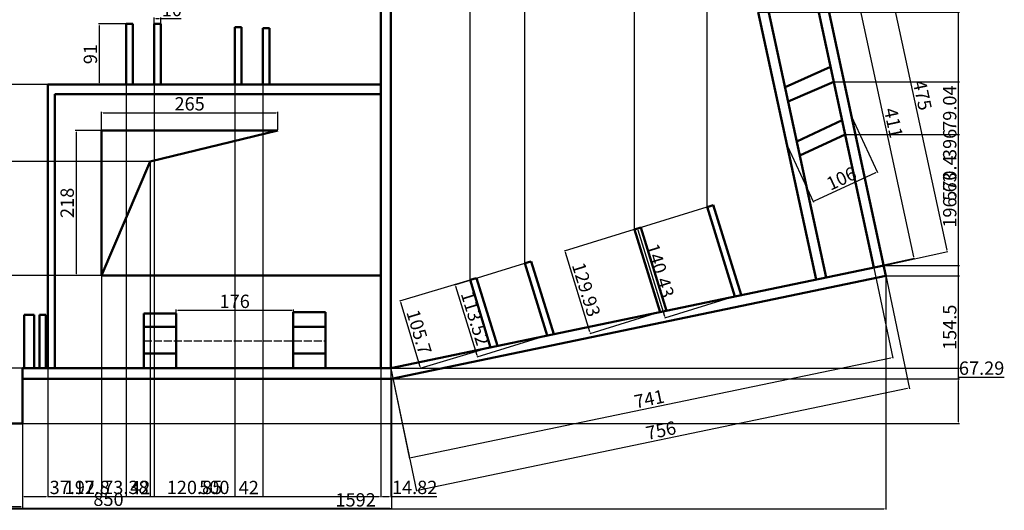
# Model space of a CAD drawing. Units: millimetres. Extents: x 1408 to 3734, y 1022 to 2569.
# Tile 2 of 3: x 2256 to 3734, y 1022 to 1758. Entities that reach past the tile are written whole.
import ezdxf

# ---------------------------------------------------------------- set-up
doc = ezdxf.new("R2010")
doc.units = ezdxf.units.MM
doc.linetypes.add('ACAD_ISO02W100', pattern=[15, 12, -3])
for name, color, linetype, lineweight in [('M-DIMS', 2, 'Continuous', 25), ('M-HIDN', 4, 'ACAD_ISO02W100', 25), ('M-OUTL', 7, 'Continuous', 50)]:
    doc.layers.add(name, color=color, linetype=linetype, lineweight=lineweight)
doc.styles.get("Standard").update_dxf_attribs({"font": 'arial.ttf'})
doc.dimstyles.new('ISO-25', dxfattribs={"dimtxt": 20, "dimasz": 2.5, "dimexe": 1.25, "dimexo": 0.625, "dimtad": 1, "dimtoh": 1, "dimdec": 0, "dimtxsty": 'Standard', "dimcen": 2.5, "dimadec": 0, "dimazin": 0, "dimtfac": 1, "dimtdec": 0, "dimtmove": 0, "dimatfit": 3, "dimfxl": 1, "dimarcsym": 0})

# ---------------------------------------------------------------- blocks, each defined once
blk = doc.blocks.new('*D6')
at = {"layer": 'Defpoints', "color": 0, "transparency": 16777216}
for p in [(1964.7, 1152.1), (2260.7, 1152.1), (2260.7, 1027.5)]:
    blk.add_point(p, dxfattribs=at)
at = {"layer": 'M-DIMS', "color": 0, "lineweight": -2, "transparency": 16777216}
for p, q in [((1964.7, 1151.5), (1964.7, 1026.2)), ((2260.7, 1151.5), (2260.7, 1026.2)), ((1967.2, 1027.5), (2258.2, 1027.5))]:
    blk.add_line(p, q, dxfattribs=at)
at = {"layer": 'M-DIMS', "color": 0, "transparency": 16777216}
for points in [[(1967.2, 1027.9), (1967.2, 1027.1), (1964.7, 1027.5)], [(2258.2, 1027.9), (2258.2, 1027.1), (2260.7, 1027.5)]]:
    blk.add_solid(points, dxfattribs=at)
at = {"layer": 'M-DIMS', "color": 0, "transparency": 16777216, "insert": (2112.7, 1038.3), "char_height": 20, "attachment_point": 5}
blk.add_mtext('296', dxfattribs=at)
blk = doc.blocks.new('*D7')
at = {"layer": 'Defpoints', "color": 0, "transparency": 16777216}
for p in [(2814.7, 1219.4), (1964.7, 1152.1), (2814.7, 1025)]:
    blk.add_point(p, dxfattribs=at)
at = {"layer": 'M-DIMS', "color": 0, "lineweight": -2, "transparency": 16777216}
for p, q in [((2814.7, 1218.8), (2814.7, 1023.8)), ((1964.7, 1151.5), (1964.7, 1023.8)), ((1967.2, 1025), (2812.2, 1025))]:
    blk.add_line(p, q, dxfattribs=at)
at = {"layer": 'M-DIMS', "color": 0, "transparency": 16777216}
for points in [[(1967.2, 1025.5), (1967.2, 1024.6), (1964.7, 1025)], [(2812.2, 1025.5), (2812.2, 1024.6), (2814.7, 1025)]]:
    blk.add_solid(points, dxfattribs=at)
at = {"layer": 'M-DIMS', "color": 0, "transparency": 16777216, "insert": (2389.7, 1035.9), "char_height": 20, "attachment_point": 5}
blk.add_mtext('850', dxfattribs=at)
blk = doc.blocks.new('*D8')
at = {"layer": 'Defpoints', "color": 0, "transparency": 16777216}
for p in [(3556.7, 1373.9), (1964.7, 1152.1), (3556.7, 1024.2)]:
    blk.add_point(p, dxfattribs=at)
at = {"layer": 'M-DIMS', "color": 0, "lineweight": -2, "transparency": 16777216}
for p, q in [((3556.7, 1373.3), (3556.7, 1022.9)), ((1964.7, 1151.5), (1964.7, 1022.9)), ((1967.2, 1024.2), (3554.2, 1024.2))]:
    blk.add_line(p, q, dxfattribs=at)
at = {"layer": 'M-DIMS', "color": 0, "transparency": 16777216}
for points in [[(1967.2, 1024.6), (1967.2, 1023.8), (1964.7, 1024.2)], [(3554.2, 1024.6), (3554.2, 1023.8), (3556.7, 1024.2)]]:
    blk.add_solid(points, dxfattribs=at)
at = {"layer": 'M-DIMS', "color": 0, "transparency": 16777216, "insert": (2760.7, 1035), "char_height": 20, "attachment_point": 5}
blk.add_mtext('1592', dxfattribs=at)
blk = doc.blocks.new('*D12')
at = {"layer": 'Defpoints', "color": 0, "transparency": 16777216}
for p in [(3453.1, 1853.8), (3648.6, 1410), (3553.5, 1389.5)]:
    blk.add_point(p, dxfattribs=at)
at = {"layer": 'M-DIMS', "color": 0, "lineweight": -2, "transparency": 16777216}
for p, q in [((3453.7, 1854), (3549.5, 1874.7)), ((3548.8, 1871.9), (3648.1, 1412.5)), ((3554.1, 1389.6), (3649.8, 1410.3))]:
    blk.add_line(p, q, dxfattribs=at)
at = {"layer": 'M-DIMS', "color": 0, "transparency": 16777216}
for points in [[(3549.2, 1872), (3548.4, 1871.9), (3548.3, 1874.4)], [(3648.5, 1412.6), (3647.7, 1412.4), (3648.6, 1410)]]:
    blk.add_solid(points, dxfattribs=at)
at = {"layer": 'M-DIMS', "color": 0, "transparency": 16777216, "insert": (3609, 1644.5), "char_height": 20, "attachment_point": 5, "rotation": 282.1929}
blk.add_mtext('475', dxfattribs=at)
blk = doc.blocks.new('*D14')
at = {"layer": 'Defpoints', "color": 0, "transparency": 16777216}
for p in [(2416.4, 1752.1), (2375.9, 1661.3), (2416.4, 1661.3)]:
    blk.add_point(p, dxfattribs=at)
at = {"layer": 'M-DIMS', "color": 0, "lineweight": -2, "transparency": 16777216}
for p, q in [((2415.8, 1752.1), (2374.7, 1752.1)), ((2375.9, 1749.6), (2375.9, 1663.8)), ((2415.8, 1661.3), (2374.7, 1661.3))]:
    blk.add_line(p, q, dxfattribs=at)
at = {"layer": 'M-DIMS', "color": 0, "transparency": 16777216}
for points in [[(2375.5, 1749.6), (2376.3, 1749.6), (2375.9, 1752.1)], [(2375.5, 1663.8), (2376.3, 1663.8), (2375.9, 1661.3)]]:
    blk.add_solid(points, dxfattribs=at)
at = {"layer": 'M-DIMS', "color": 0, "transparency": 16777216, "insert": (2365.1, 1706.7), "char_height": 20, "attachment_point": 5, "rotation": 90}
blk.add_mtext('91', dxfattribs=at)
blk = doc.blocks.new('*D15')
at = {"layer": 'Defpoints', "color": 0, "transparency": 16777216}
for p in [(2468.4, 1760.2), (2458.4, 1752.1), (2468.4, 1752.1)]:
    blk.add_point(p, dxfattribs=at)
at = {"layer": 'M-DIMS', "color": 0, "lineweight": -2, "transparency": 16777216}
for p, q in [((2458.4, 1752.7), (2458.4, 1761.5)), ((2460.9, 1760.2), (2465.9, 1760.2)), ((2468.4, 1752.7), (2468.4, 1761.5)), ((2468.4, 1760.2), (2498.9, 1760.2))]:
    blk.add_line(p, q, dxfattribs=at)
at = {"layer": 'M-DIMS', "color": 0, "transparency": 16777216}
for points in [[(2460.9, 1760.6), (2460.9, 1759.8), (2458.4, 1760.2)], [(2465.9, 1760.6), (2465.9, 1759.8), (2468.4, 1760.2)]]:
    blk.add_solid(points, dxfattribs=at)
at = {"layer": 'M-DIMS', "color": 0, "transparency": 16777216, "insert": (2484.9, 1771), "char_height": 20, "attachment_point": 5}
blk.add_mtext('10', dxfattribs=at)
blk = doc.blocks.new('*D16')
at = {"layer": 'Defpoints', "color": 0, "transparency": 16777216}
for p in [(2644, 1618.7), (2379.1, 1592.2), (2644, 1592.2)]:
    blk.add_point(p, dxfattribs=at)
at = {"layer": 'M-DIMS', "color": 0, "lineweight": -2, "transparency": 16777216}
for p, q in [((2379.1, 1592.9), (2379.1, 1620)), ((2381.6, 1618.7), (2641.5, 1618.7)), ((2644, 1592.9), (2644, 1620))]:
    blk.add_line(p, q, dxfattribs=at)
at = {"layer": 'M-DIMS', "color": 0, "transparency": 16777216}
for points in [[(2381.6, 1619.1), (2381.6, 1618.3), (2379.1, 1618.7)], [(2641.5, 1619.1), (2641.5, 1618.3), (2644, 1618.7)]]:
    blk.add_solid(points, dxfattribs=at)
at = {"layer": 'M-DIMS', "color": 0, "transparency": 16777216, "insert": (2511.5, 1629.5), "char_height": 20, "attachment_point": 5}
blk.add_mtext('265', dxfattribs=at)
blk = doc.blocks.new('*D17')
at = {"layer": 'Defpoints', "color": 0, "transparency": 16777216}
for p in [(2379.1, 1592.2), (2341.1, 1374.6), (2379.1, 1374.6)]:
    blk.add_point(p, dxfattribs=at)
at = {"layer": 'M-DIMS', "color": 0, "lineweight": -2, "transparency": 16777216}
for p, q in [((2378.5, 1592.2), (2339.9, 1592.2)), ((2341.1, 1589.7), (2341.1, 1377.1)), ((2378.5, 1374.6), (2339.9, 1374.6))]:
    blk.add_line(p, q, dxfattribs=at)
at = {"layer": 'M-DIMS', "color": 0, "transparency": 16777216}
for points in [[(2340.7, 1589.7), (2341.5, 1589.7), (2341.1, 1592.2)], [(2340.7, 1377.1), (2341.5, 1377.1), (2341.1, 1374.6)]]:
    blk.add_solid(points, dxfattribs=at)
at = {"layer": 'M-DIMS', "color": 0, "transparency": 16777216, "insert": (2330.3, 1483.4), "char_height": 20, "attachment_point": 5, "rotation": 90}
blk.add_mtext('218', dxfattribs=at)
blk = doc.blocks.new('*D26')
at = {"layer": 'Defpoints', "color": 0, "transparency": 16777216}
for p in [(3538.7, 1386.4), (3566.8, 1251.5), (2813.4, 1235.4)]:
    blk.add_point(p, dxfattribs=at)
at = {"layer": 'M-DIMS', "color": 0, "lineweight": -2, "transparency": 16777216}
for p, q in [((3538.8, 1385.8), (3567, 1250.3)), ((2844, 1101), (3564.3, 1251)), ((2813.6, 1234.8), (2841.8, 1099.3))]:
    blk.add_line(p, q, dxfattribs=at)
at = {"layer": 'M-DIMS', "color": 0, "transparency": 16777216}
for points in [[(3564.2, 1251.4), (3564.4, 1250.6), (3566.8, 1251.5)], [(2843.9, 1101.4), (2844, 1100.6), (2841.5, 1100.5)]]:
    blk.add_solid(points, dxfattribs=at)
at = {"layer": 'M-DIMS', "color": 0, "transparency": 16777216, "insert": (3202, 1186.5), "char_height": 20, "attachment_point": 5, "rotation": 11.7622}
blk.add_mtext('741', dxfattribs=at)
blk = doc.blocks.new('*D28')
at = {"layer": 'Defpoints', "color": 0, "transparency": 16777216}
for p in [(3365.2, 1769.9), (3598.5, 1400), (3451.8, 1368.3)]:
    blk.add_point(p, dxfattribs=at)
at = {"layer": 'M-DIMS', "color": 0, "lineweight": -2, "transparency": 16777216}
for p, q in [((3365.8, 1770), (3513.1, 1801.8)), ((3512.4, 1799.1), (3598, 1402.4)), ((3452.4, 1368.4), (3599.8, 1400.2))]:
    blk.add_line(p, q, dxfattribs=at)
at = {"layer": 'M-DIMS', "color": 0, "transparency": 16777216}
for points in [[(3512.8, 1799.2), (3512, 1799), (3511.9, 1801.5)], [(3598.4, 1402.5), (3597.6, 1402.3), (3598.5, 1400)]]:
    blk.add_solid(points, dxfattribs=at)
at = {"layer": 'M-DIMS', "color": 0, "transparency": 16777216, "insert": (3565.6, 1603), "char_height": 20, "attachment_point": 5, "rotation": 282.179}
blk.add_mtext('411', dxfattribs=at)
blk = doc.blocks.new('*D29')
at = {"layer": 'Defpoints', "color": 0, "transparency": 16777216}
for p in [(3553.5, 1389.5), (2813.4, 1235.4), (3591.7, 1205.7)]:
    blk.add_point(p, dxfattribs=at)
at = {"layer": 'M-DIMS', "color": 0, "lineweight": -2, "transparency": 16777216}
for p, q in [((3553.6, 1388.9), (3592, 1204.5)), ((2813.6, 1234.8), (2852, 1050.4)), ((2854.1, 1052.1), (3589.3, 1205.2))]:
    blk.add_line(p, q, dxfattribs=at)
at = {"layer": 'M-DIMS', "color": 0, "transparency": 16777216}
for points in [[(3589.2, 1205.6), (3589.4, 1204.8), (3591.7, 1205.7)], [(2854.1, 1052.5), (2854.2, 1051.7), (2851.7, 1051.6)]]:
    blk.add_solid(points, dxfattribs=at)
at = {"layer": 'M-DIMS', "color": 0, "transparency": 16777216, "insert": (3219.5, 1139.3), "char_height": 20, "attachment_point": 5, "rotation": 11.7622}
blk.add_mtext('756', dxfattribs=at)
blk = doc.blocks.new('*D38')
at = {"layer": 'Defpoints', "color": 0, "transparency": 16777216}
for p in [(3504.9, 1613.9), (3408.5, 1569.1), (3543.7, 1530.2)]:
    blk.add_point(p, dxfattribs=at)
at = {"layer": 'M-DIMS', "color": 0, "lineweight": -2, "transparency": 16777216}
for p, q in [((3505.2, 1613.3), (3544.3, 1529.1)), ((3408.8, 1568.5), (3447.8, 1484.3)), ((3449.6, 1486.5), (3541.5, 1529.2))]:
    blk.add_line(p, q, dxfattribs=at)
at = {"layer": 'M-DIMS', "color": 0, "transparency": 16777216}
for points in [[(3541.3, 1529.5), (3541.6, 1528.8), (3543.7, 1530.2)], [(3449.4, 1486.9), (3449.8, 1486.1), (3447.3, 1485.5)]]:
    blk.add_solid(points, dxfattribs=at)
at = {"layer": 'M-DIMS', "color": 0, "transparency": 16777216, "insert": (3491, 1517.7), "char_height": 20, "attachment_point": 5, "rotation": 24.905}
blk.add_mtext('106', dxfattribs=at)
blk = doc.blocks.new('*D39')
at = {"layer": 'Defpoints', "color": 0, "transparency": 16777216}
for p in [(2667.2, 1322.2), (2491.1, 1276.3), (2667.2, 1277.4)]:
    blk.add_point(p, dxfattribs=at)
at = {"layer": 'M-DIMS', "color": 0, "lineweight": -2, "transparency": 16777216}
for p, q in [((2491.1, 1276.9), (2491.1, 1323.4)), ((2493.6, 1322.2), (2664.7, 1322.2)), ((2667.2, 1278), (2667.2, 1323.4))]:
    blk.add_line(p, q, dxfattribs=at)
at = {"layer": 'M-DIMS', "color": 0, "transparency": 16777216}
for points in [[(2493.6, 1322.6), (2493.6, 1321.8), (2491.1, 1322.2)], [(2664.7, 1322.6), (2664.7, 1321.8), (2667.2, 1322.2)]]:
    blk.add_solid(points, dxfattribs=at)
at = {"layer": 'M-DIMS', "color": 0, "transparency": 16777216, "insert": (2579.2, 1333), "char_height": 20, "attachment_point": 5}
blk.add_mtext('176', dxfattribs=at)
blk = doc.blocks.new('*D51')
at = {"layer": 'Defpoints', "color": 0, "transparency": 16777216}
for p in [(3365.2, 1769.9), (3665.9, 1769.9), (3556.7, 1373.9)]:
    blk.add_point(p, dxfattribs=at)
at = {"layer": 'M-DIMS', "color": 0, "lineweight": -2, "transparency": 16777216}
for p, q in [((3365.8, 1769.9), (3667.2, 1769.9)), ((3665.9, 1376.4), (3665.9, 1767.4)), ((3557.3, 1373.9), (3667.2, 1373.9))]:
    blk.add_line(p, q, dxfattribs=at)
at = {"layer": 'M-DIMS', "color": 0, "transparency": 16777216}
for points in [[(3665.5, 1767.4), (3666.4, 1767.4), (3665.9, 1769.9)], [(3665.5, 1376.4), (3666.4, 1376.4), (3665.9, 1373.9)]]:
    blk.add_solid(points, dxfattribs=at)
at = {"layer": 'M-DIMS', "color": 0, "transparency": 16777216, "insert": (3655.1, 1571.9), "char_height": 20, "attachment_point": 5, "rotation": 90}
blk.add_mtext('396', dxfattribs=at)
blk = doc.blocks.new('*D53')
at = {"layer": 'Defpoints', "color": 0, "transparency": 16777216}
for p in [(3556.7, 1373.9), (3665.9, 1373.9), (2814.7, 1219.4)]:
    blk.add_point(p, dxfattribs=at)
at = {"layer": 'M-DIMS', "color": 0, "lineweight": -2, "transparency": 16777216}
for p, q in [((3557.3, 1373.9), (3667.2, 1373.9)), ((3665.9, 1221.9), (3665.9, 1371.4)), ((2815.3, 1219.4), (3667.2, 1219.4))]:
    blk.add_line(p, q, dxfattribs=at)
at = {"layer": 'M-DIMS', "color": 0, "transparency": 16777216}
for points in [[(3665.5, 1371.4), (3666.4, 1371.4), (3665.9, 1373.9)], [(3665.5, 1221.9), (3666.4, 1221.9), (3665.9, 1219.4)]]:
    blk.add_solid(points, dxfattribs=at)
at = {"layer": 'M-DIMS', "color": 0, "transparency": 16777216, "insert": (3655.1, 1296.6), "char_height": 20, "attachment_point": 5, "rotation": 90}
blk.add_mtext('154.5', dxfattribs=at)
blk = doc.blocks.new('*D54')
at = {"layer": 'Defpoints', "color": 0, "transparency": 16777216}
for p in [(2260.7, 1219.4), (3665.9, 1219.4), (2260.7, 1152.1)]:
    blk.add_point(p, dxfattribs=at)
at = {"layer": 'M-DIMS', "color": 0, "lineweight": -2, "transparency": 16777216}
for p, q in [((2261.3, 1219.4), (3667.2, 1219.4)), ((3665.9, 1219.4), (3665.9, 1221.9)), ((3665.9, 1221.9), (3734.2, 1221.9)), ((3665.9, 1154.6), (3665.9, 1216.9)), ((2261.3, 1152.1), (3667.2, 1152.1))]:
    blk.add_line(p, q, dxfattribs=at)
at = {"layer": 'M-DIMS', "color": 0, "transparency": 16777216}
for points in [[(3665.5, 1216.9), (3666.4, 1216.9), (3665.9, 1219.4)], [(3665.5, 1154.6), (3666.4, 1154.6), (3665.9, 1152.1)]]:
    blk.add_solid(points, dxfattribs=at)
at = {"layer": 'M-DIMS', "color": 0, "transparency": 16777216, "insert": (3700.4, 1232.7), "char_height": 20, "attachment_point": 5}
blk.add_mtext('67.29', dxfattribs=at)
blk = doc.blocks.new('*D55')
at = {"layer": 'Defpoints', "color": 0, "transparency": 16777216}
for p in [(2298.6, 1661.3), (2260.7, 1219.4), (2298.6, 1042.8)]:
    blk.add_point(p, dxfattribs=at)
at = {"layer": 'M-DIMS', "color": 0, "lineweight": -2, "transparency": 16777216}
for p, q in [((2298.6, 1660.6), (2298.6, 1041.6)), ((2260.7, 1218.8), (2260.7, 1041.6)), ((2263.2, 1042.8), (2296.1, 1042.8)), ((2298.6, 1042.8), (2369.6, 1042.8))]:
    blk.add_line(p, q, dxfattribs=at)
at = {"layer": 'M-DIMS', "color": 0, "transparency": 16777216}
for points in [[(2263.2, 1043.3), (2263.2, 1042.4), (2260.7, 1042.8)], [(2296.1, 1043.3), (2296.1, 1042.4), (2298.6, 1042.8)]]:
    blk.add_solid(points, dxfattribs=at)
at = {"layer": 'M-DIMS', "color": 0, "transparency": 16777216, "insert": (2335.4, 1053.7), "char_height": 20, "attachment_point": 5}
blk.add_mtext('37.92', dxfattribs=at)
blk = doc.blocks.new('*D56')
at = {"layer": 'Defpoints', "color": 0, "transparency": 16777216}
for p in [(2798.6, 1805.8), (3665.9, 1805.8), (2813.4, 1235.4)]:
    blk.add_point(p, dxfattribs=at)
at = {"layer": 'M-DIMS', "color": 0, "lineweight": -2, "transparency": 16777216}
for p, q in [((2799.2, 1805.8), (3667.2, 1805.8)), ((3665.9, 1237.9), (3665.9, 1803.3)), ((2814.1, 1235.4), (3667.2, 1235.4))]:
    blk.add_line(p, q, dxfattribs=at)
at = {"layer": 'M-DIMS', "color": 0, "transparency": 16777216}
for points in [[(3665.5, 1803.3), (3666.4, 1803.3), (3665.9, 1805.8)], [(3665.5, 1237.9), (3666.4, 1237.9), (3665.9, 1235.4)]]:
    blk.add_solid(points, dxfattribs=at)
at = {"layer": 'M-DIMS', "color": 0, "transparency": 16777216, "insert": (3655.1, 1520.6), "char_height": 20, "attachment_point": 5, "rotation": 90}
blk.add_mtext('570.4', dxfattribs=at)
blk = doc.blocks.new('*D58')
at = {"layer": 'Defpoints', "color": 0, "transparency": 16777216}
for p in [(2798.6, 1661.3), (2813.4, 1235.4), (2813.4, 1042.8)]:
    blk.add_point(p, dxfattribs=at)
at = {"layer": 'M-DIMS', "color": 0, "lineweight": -2, "transparency": 16777216}
for p, q in [((2798.6, 1660.6), (2798.6, 1041.6)), ((2813.4, 1234.8), (2813.4, 1041.6)), ((2801.1, 1042.8), (2810.9, 1042.8)), ((2813.4, 1042.8), (2882.6, 1042.8))]:
    blk.add_line(p, q, dxfattribs=at)
at = {"layer": 'M-DIMS', "color": 0, "transparency": 16777216}
for points in [[(2801.1, 1043.3), (2801.1, 1042.4), (2798.6, 1042.8)], [(2810.9, 1043.3), (2810.9, 1042.4), (2813.4, 1042.8)]]:
    blk.add_solid(points, dxfattribs=at)
at = {"layer": 'M-DIMS', "color": 0, "transparency": 16777216, "insert": (2849.3, 1053.7), "char_height": 20, "attachment_point": 5}
blk.add_mtext('14.82', dxfattribs=at)
blk = doc.blocks.new('*D59')
at = {"layer": 'Defpoints', "color": 0, "transparency": 16777216}
for p in [(2298.6, 1661.3), (2798.6, 1661.3), (2798.6, 1042.8)]:
    blk.add_point(p, dxfattribs=at)
at = {"layer": 'M-DIMS', "color": 0, "lineweight": -2, "transparency": 16777216}
for p, q in [((2298.6, 1660.6), (2298.6, 1041.6)), ((2798.6, 1660.6), (2798.6, 1041.6)), ((2301.1, 1042.8), (2796.1, 1042.8))]:
    blk.add_line(p, q, dxfattribs=at)
at = {"layer": 'M-DIMS', "color": 0, "transparency": 16777216}
for points in [[(2301.1, 1043.3), (2301.1, 1042.4), (2298.6, 1042.8)], [(2796.1, 1043.3), (2796.1, 1042.4), (2798.6, 1042.8)]]:
    blk.add_solid(points, dxfattribs=at)
at = {"layer": 'M-DIMS', "color": 0, "transparency": 16777216, "insert": (2548.6, 1053.7), "char_height": 20, "attachment_point": 5}
blk.add_mtext('500', dxfattribs=at)
blk = doc.blocks.new('*D60')
at = {"layer": 'Defpoints', "color": 0, "transparency": 16777216}
for p in [(1475.7, 1661.3), (2298.6, 1661.3), (2298.6, 1235.4)]:
    blk.add_point(p, dxfattribs=at)
at = {"layer": 'M-DIMS', "color": 0, "lineweight": -2, "transparency": 16777216}
for p, q in [((2298, 1661.3), (1474.5, 1661.3)), ((1475.7, 1237.9), (1475.7, 1658.8)), ((2298, 1235.4), (1474.5, 1235.4))]:
    blk.add_line(p, q, dxfattribs=at)
at = {"layer": 'M-DIMS', "color": 0, "transparency": 16777216}
for points in [[(1475.3, 1658.8), (1476.1, 1658.8), (1475.7, 1661.3)], [(1475.3, 1237.9), (1476.1, 1237.9), (1475.7, 1235.4)]]:
    blk.add_solid(points, dxfattribs=at)
at = {"layer": 'M-DIMS', "color": 0, "transparency": 16777216, "insert": (1464.9, 1448.3), "char_height": 20, "attachment_point": 5, "rotation": 90}
blk.add_mtext('425.9', dxfattribs=at)
blk = doc.blocks.new('*D61')
at = {"layer": 'Defpoints', "color": 0, "transparency": 16777216}
for p in [(2452.5, 1545.3), (2379.1, 1374.6), (2452.5, 1042.8)]:
    blk.add_point(p, dxfattribs=at)
at = {"layer": 'M-DIMS', "color": 0, "lineweight": -2, "transparency": 16777216}
for p, q in [((2452.5, 1544.6), (2452.5, 1041.6)), ((2379.1, 1373.9), (2379.1, 1041.6)), ((2381.6, 1042.8), (2450, 1042.8))]:
    blk.add_line(p, q, dxfattribs=at)
at = {"layer": 'M-DIMS', "color": 0, "transparency": 16777216}
for points in [[(2381.6, 1043.3), (2381.6, 1042.4), (2379.1, 1042.8)], [(2450, 1043.3), (2450, 1042.4), (2452.5, 1042.8)]]:
    blk.add_solid(points, dxfattribs=at)
at = {"layer": 'M-DIMS', "color": 0, "transparency": 16777216, "insert": (2415.8, 1053.7), "char_height": 20, "attachment_point": 5}
blk.add_mtext('73.38', dxfattribs=at)
blk = doc.blocks.new('*D62')
at = {"layer": 'Defpoints', "color": 0, "transparency": 16777216}
for p in [(1475.7, 1545.3), (2452.5, 1545.3), (2379.1, 1374.6)]:
    blk.add_point(p, dxfattribs=at)
at = {"layer": 'M-DIMS', "color": 0, "lineweight": -2, "transparency": 16777216}
for p, q in [((2451.8, 1545.3), (1474.5, 1545.3)), ((1475.7, 1377.1), (1475.7, 1542.8)), ((2378.5, 1374.6), (1474.5, 1374.6))]:
    blk.add_line(p, q, dxfattribs=at)
at = {"layer": 'M-DIMS', "color": 0, "transparency": 16777216}
for points in [[(1475.3, 1542.8), (1476.1, 1542.8), (1475.7, 1545.3)], [(1475.3, 1377.1), (1476.1, 1377.1), (1475.7, 1374.6)]]:
    blk.add_solid(points, dxfattribs=at)
at = {"layer": 'M-DIMS', "color": 0, "transparency": 16777216, "insert": (1464.9, 1459.9), "char_height": 20, "attachment_point": 5, "rotation": 90}
blk.add_mtext('170.7', dxfattribs=at)
blk = doc.blocks.new('*D63')
at = {"layer": 'Defpoints', "color": 0, "transparency": 16777216}
for p in [(2416.4, 1752.1), (2298.6, 1661.3), (2416.4, 1042.8)]:
    blk.add_point(p, dxfattribs=at)
at = {"layer": 'M-DIMS', "color": 0, "lineweight": -2, "transparency": 16777216}
for p, q in [((2416.4, 1751.5), (2416.4, 1041.6)), ((2298.6, 1660.6), (2298.6, 1041.6)), ((2301.1, 1042.8), (2413.9, 1042.8))]:
    blk.add_line(p, q, dxfattribs=at)
at = {"layer": 'M-DIMS', "color": 0, "transparency": 16777216}
for points in [[(2301.1, 1043.3), (2301.1, 1042.4), (2298.6, 1042.8)], [(2413.9, 1043.3), (2413.9, 1042.4), (2416.4, 1042.8)]]:
    blk.add_solid(points, dxfattribs=at)
at = {"layer": 'M-DIMS', "color": 0, "transparency": 16777216, "insert": (2357.5, 1053.7), "char_height": 20, "attachment_point": 5}
blk.add_mtext('117.8', dxfattribs=at)
blk = doc.blocks.new('*D64')
at = {"layer": 'Defpoints', "color": 0, "transparency": 16777216}
for p in [(2416.4, 1752.1), (2458.4, 1752.1), (2458.4, 1042.8)]:
    blk.add_point(p, dxfattribs=at)
at = {"layer": 'M-DIMS', "color": 0, "lineweight": -2, "transparency": 16777216}
for p, q in [((2416.4, 1751.5), (2416.4, 1041.6)), ((2458.4, 1751.5), (2458.4, 1041.6)), ((2418.9, 1042.8), (2455.9, 1042.8))]:
    blk.add_line(p, q, dxfattribs=at)
at = {"layer": 'M-DIMS', "color": 0, "transparency": 16777216}
for points in [[(2418.9, 1043.3), (2418.9, 1042.4), (2416.4, 1042.8)], [(2455.9, 1043.3), (2455.9, 1042.4), (2458.4, 1042.8)]]:
    blk.add_solid(points, dxfattribs=at)
at = {"layer": 'M-DIMS', "color": 0, "transparency": 16777216, "insert": (2437.4, 1053.5), "char_height": 20, "attachment_point": 5}
blk.add_mtext('42', dxfattribs=at)
blk = doc.blocks.new('*D65')
at = {"layer": 'Defpoints', "color": 0, "transparency": 16777216}
for p in [(2458.4, 1752.1), (2579.3, 1747), (2579.3, 1042.8)]:
    blk.add_point(p, dxfattribs=at)
at = {"layer": 'M-DIMS', "color": 0, "lineweight": -2, "transparency": 16777216}
for p, q in [((2458.4, 1751.5), (2458.4, 1041.6)), ((2579.3, 1746.4), (2579.3, 1041.6)), ((2460.9, 1042.8), (2576.8, 1042.8))]:
    blk.add_line(p, q, dxfattribs=at)
at = {"layer": 'M-DIMS', "color": 0, "transparency": 16777216}
for points in [[(2460.9, 1043.3), (2460.9, 1042.4), (2458.4, 1042.8)], [(2576.8, 1043.3), (2576.8, 1042.4), (2579.3, 1042.8)]]:
    blk.add_solid(points, dxfattribs=at)
at = {"layer": 'M-DIMS', "color": 0, "transparency": 16777216, "insert": (2518.8, 1053.7), "char_height": 20, "attachment_point": 5}
blk.add_mtext('120.85', dxfattribs=at)
blk = doc.blocks.new('*D66')
at = {"layer": 'Defpoints', "color": 0, "transparency": 16777216}
for p in [(2579.3, 1747), (2621.3, 1745.8), (2621.3, 1042.8)]:
    blk.add_point(p, dxfattribs=at)
at = {"layer": 'M-DIMS', "color": 0, "lineweight": -2, "transparency": 16777216}
for p, q in [((2579.3, 1746.4), (2579.3, 1041.6)), ((2621.3, 1745.1), (2621.3, 1041.6)), ((2581.8, 1042.8), (2618.8, 1042.8))]:
    blk.add_line(p, q, dxfattribs=at)
at = {"layer": 'M-DIMS', "color": 0, "transparency": 16777216}
for points in [[(2581.8, 1043.3), (2581.8, 1042.4), (2579.3, 1042.8)], [(2618.8, 1043.3), (2618.8, 1042.4), (2621.3, 1042.8)]]:
    blk.add_solid(points, dxfattribs=at)
at = {"layer": 'M-DIMS', "color": 0, "transparency": 16777216, "insert": (2600.3, 1053.5), "char_height": 20, "attachment_point": 5}
blk.add_mtext('42', dxfattribs=at)
blk = doc.blocks.new('*D75')
at = {"layer": 'Defpoints', "color": 0, "transparency": 16777216}
for p in [(3495.6, 1586.1), (3665.9, 1586.1), (3553.5, 1389.5)]:
    blk.add_point(p, dxfattribs=at)
at = {"layer": 'M-DIMS', "color": 0, "lineweight": -2, "transparency": 16777216}
for p, q in [((3496.2, 1586.1), (3667.2, 1586.1)), ((3665.9, 1392), (3665.9, 1583.6)), ((3554.1, 1389.5), (3667.2, 1389.5))]:
    blk.add_line(p, q, dxfattribs=at)
at = {"layer": 'M-DIMS', "color": 0, "transparency": 16777216}
for points in [[(3665.5, 1583.6), (3666.4, 1583.6), (3665.9, 1586.1)], [(3665.5, 1392), (3666.4, 1392), (3665.9, 1389.5)]]:
    blk.add_solid(points, dxfattribs=at)
at = {"layer": 'M-DIMS', "color": 0, "transparency": 16777216, "insert": (3655.1, 1487.8), "char_height": 20, "attachment_point": 5, "rotation": 90}
blk.add_mtext('196.63', dxfattribs=at)
blk = doc.blocks.new('*D76')
at = {"layer": 'Defpoints', "color": 0, "transparency": 16777216}
for p in [(3478.5, 1665.1), (3665.9, 1665.1), (3495.6, 1586.1)]:
    blk.add_point(p, dxfattribs=at)
at = {"layer": 'M-DIMS', "color": 0, "lineweight": -2, "transparency": 16777216}
for p, q in [((3479.2, 1665.1), (3667.2, 1665.1)), ((3665.9, 1588.6), (3665.9, 1662.6)), ((3496.2, 1586.1), (3667.2, 1586.1))]:
    blk.add_line(p, q, dxfattribs=at)
at = {"layer": 'M-DIMS', "color": 0, "transparency": 16777216}
for points in [[(3665.5, 1662.6), (3666.4, 1662.6), (3665.9, 1665.1)], [(3665.5, 1588.6), (3666.4, 1588.6), (3665.9, 1586.1)]]:
    blk.add_solid(points, dxfattribs=at)
at = {"layer": 'M-DIMS', "color": 0, "transparency": 16777216, "insert": (3655.1, 1625.6), "char_height": 20, "attachment_point": 5, "rotation": 90}
blk.add_mtext('79.04', dxfattribs=at)
blk = doc.blocks.new('*D77')
at = {"layer": 'Defpoints', "color": 0, "transparency": 16777216}
for p in [(2932.6, 2544.6), (2932.6, 1367.8), (2813.4, 1235.4)]:
    blk.add_point(p, dxfattribs=at)
at = {"layer": 'M-DIMS', "color": 0, "lineweight": -2, "transparency": 16777216}
for p, q in [((2813.4, 1236), (2813.4, 2545.9)), ((2815.9, 2544.6), (2930.1, 2544.6)), ((2932.6, 1368.4), (2932.6, 2545.9))]:
    blk.add_line(p, q, dxfattribs=at)
at = {"layer": 'M-DIMS', "color": 0, "transparency": 16777216}
for points in [[(2815.9, 2545), (2815.9, 2544.2), (2813.4, 2544.6)], [(2930.1, 2545), (2930.1, 2544.2), (2932.6, 2544.6)]]:
    blk.add_solid(points, dxfattribs=at)
at = {"layer": 'M-DIMS', "color": 0, "transparency": 16777216, "insert": (2873, 2555.5), "char_height": 20, "attachment_point": 5}
blk.add_mtext('119.15', dxfattribs=at)
blk = doc.blocks.new('*D78')
at = {"layer": 'Defpoints', "color": 0, "transparency": 16777216}
for p in [(3014.9, 2544.6), (3014.9, 1392.8), (2932.6, 1367.8)]:
    blk.add_point(p, dxfattribs=at)
at = {"layer": 'M-DIMS', "color": 0, "lineweight": -2, "transparency": 16777216}
for p, q in [((2932.6, 1368.4), (2932.6, 2545.9)), ((2935.1, 2544.6), (3012.4, 2544.6)), ((3014.9, 1393.4), (3014.9, 2545.9))]:
    blk.add_line(p, q, dxfattribs=at)
at = {"layer": 'M-DIMS', "color": 0, "transparency": 16777216}
for points in [[(2935.1, 2545), (2935.1, 2544.2), (2932.6, 2544.6)], [(3012.4, 2545), (3012.4, 2544.2), (3014.9, 2544.6)]]:
    blk.add_solid(points, dxfattribs=at)
at = {"layer": 'M-DIMS', "color": 0, "transparency": 16777216, "insert": (2973.7, 2555.5), "char_height": 20, "attachment_point": 5}
blk.add_mtext('82.29', dxfattribs=at)
blk = doc.blocks.new('*D79')
at = {"layer": 'Defpoints', "color": 0, "transparency": 16777216}
for p in [(3179.2, 2544.6), (3179.2, 1443.7), (3014.9, 1392.8)]:
    blk.add_point(p, dxfattribs=at)
at = {"layer": 'M-DIMS', "color": 0, "lineweight": -2, "transparency": 16777216}
for p, q in [((3014.9, 1393.4), (3014.9, 2545.9)), ((3017.4, 2544.6), (3176.7, 2544.6)), ((3179.2, 1444.3), (3179.2, 2545.9))]:
    blk.add_line(p, q, dxfattribs=at)
at = {"layer": 'M-DIMS', "color": 0, "transparency": 16777216}
for points in [[(3017.4, 2545), (3017.4, 2544.2), (3014.9, 2544.6)], [(3176.7, 2545), (3176.7, 2544.2), (3179.2, 2544.6)]]:
    blk.add_solid(points, dxfattribs=at)
at = {"layer": 'M-DIMS', "color": 0, "transparency": 16777216, "insert": (3097, 2555.5), "char_height": 20, "attachment_point": 5}
blk.add_mtext('164.33', dxfattribs=at)
blk = doc.blocks.new('*D80')
at = {"layer": 'Defpoints', "color": 0, "transparency": 16777216}
for p in [(3288.4, 2544.6), (3288.4, 1477.1), (3179.2, 1443.7)]:
    blk.add_point(p, dxfattribs=at)
at = {"layer": 'M-DIMS', "color": 0, "lineweight": -2, "transparency": 16777216}
for p, q in [((3179.2, 1444.3), (3179.2, 2545.9)), ((3181.7, 2544.6), (3285.9, 2544.6)), ((3288.4, 1477.7), (3288.4, 2545.9))]:
    blk.add_line(p, q, dxfattribs=at)
at = {"layer": 'M-DIMS', "color": 0, "transparency": 16777216}
for points in [[(3181.7, 2545), (3181.7, 2544.2), (3179.2, 2544.6)], [(3285.9, 2545), (3285.9, 2544.2), (3288.4, 2544.6)]]:
    blk.add_solid(points, dxfattribs=at)
at = {"layer": 'M-DIMS', "color": 0, "transparency": 16777216, "insert": (3233.8, 2555.5), "char_height": 20, "attachment_point": 5}
blk.add_mtext('109.21', dxfattribs=at)
blk = doc.blocks.new('*D81')
at = {"layer": 'Defpoints', "color": 0, "transparency": 16777216}
for p in [(2932.6, 1367.8), (2827.9, 1336.3), (2963, 1266.5)]:
    blk.add_point(p, dxfattribs=at)
at = {"layer": 'M-DIMS', "color": 0, "lineweight": -2, "transparency": 16777216}
for p, q in [((2932, 1367.6), (2826.7, 1336)), ((2857.6, 1237.5), (2828.7, 1333.9)), ((2962.4, 1266.3), (2857.1, 1234.7))]:
    blk.add_line(p, q, dxfattribs=at)
at = {"layer": 'M-DIMS', "color": 0, "transparency": 16777216}
for points in [[(2829.1, 1334.1), (2828.3, 1333.8), (2827.9, 1336.3)], [(2858, 1237.6), (2857.2, 1237.4), (2858.3, 1235.1)]]:
    blk.add_solid(points, dxfattribs=at)
at = {"layer": 'M-DIMS', "color": 0, "transparency": 16777216, "insert": (2853.5, 1288.8), "char_height": 20, "attachment_point": 5, "rotation": 286.7131}
blk.add_mtext('105.7', dxfattribs=at)
blk = doc.blocks.new('*D82')
at = {"layer": 'Defpoints', "color": 0, "transparency": 16777216}
for p in [(3014.9, 1392.8), (2910.5, 1360.4), (3048.5, 1284.3)]:
    blk.add_point(p, dxfattribs=at)
at = {"layer": 'M-DIMS', "color": 0, "lineweight": -2, "transparency": 16777216}
for p, q in [((3014.3, 1392.6), (2909.3, 1360.1)), ((2943.4, 1254.4), (2911.3, 1358)), ((3047.9, 1284.1), (2942.9, 1251.6))]:
    blk.add_line(p, q, dxfattribs=at)
at = {"layer": 'M-DIMS', "color": 0, "transparency": 16777216}
for points in [[(2911.7, 1358.2), (2910.9, 1357.9), (2910.5, 1360.4)], [(2943.8, 1254.5), (2943, 1254.3), (2944.1, 1252)]]:
    blk.add_solid(points, dxfattribs=at)
at = {"layer": 'M-DIMS', "color": 0, "transparency": 16777216, "insert": (2937.7, 1309.4), "char_height": 20, "attachment_point": 5, "rotation": 287.2096}
blk.add_mtext('113.52', dxfattribs=at)
blk = doc.blocks.new('*D83')
at = {"layer": 'Defpoints', "color": 0, "transparency": 16777216}
for p in [(3179.2, 1443.7), (3074.8, 1411.3), (3217.6, 1319.5)]:
    blk.add_point(p, dxfattribs=at)
at = {"layer": 'M-DIMS', "color": 0, "lineweight": -2, "transparency": 16777216}
for p, q in [((3178.6, 1443.5), (3073.7, 1411)), ((3112.5, 1289.6), (3075.6, 1408.9)), ((3217, 1319.4), (3112.1, 1286.8))]:
    blk.add_line(p, q, dxfattribs=at)
at = {"layer": 'M-DIMS', "color": 0, "transparency": 16777216}
for points in [[(3076, 1409.1), (3075.2, 1408.8), (3074.8, 1411.3)], [(3112.9, 1289.7), (3112.1, 1289.5), (3113.3, 1287.2)]]:
    blk.add_solid(points, dxfattribs=at)
at = {"layer": 'M-DIMS', "color": 0, "transparency": 16777216, "insert": (3104.4, 1352.5), "char_height": 20, "attachment_point": 5, "rotation": 287.2096}
blk.add_mtext('129.93', dxfattribs=at)
blk = doc.blocks.new('*D84')
at = {"layer": 'Defpoints', "color": 0, "transparency": 16777216}
for p in [(3288.4, 1477.1), (3184.1, 1444.8), (3330, 1342.9)]:
    blk.add_point(p, dxfattribs=at)
at = {"layer": 'M-DIMS', "color": 0, "lineweight": -2, "transparency": 16777216}
for p, q in [((3287.8, 1476.9), (3182.9, 1444.4)), ((3224.9, 1313), (3184.8, 1442.4)), ((3329.4, 1342.7), (3224.4, 1310.2))]:
    blk.add_line(p, q, dxfattribs=at)
at = {"layer": 'M-DIMS', "color": 0, "transparency": 16777216}
for points in [[(3185.2, 1442.5), (3184.4, 1442.2), (3184.1, 1444.8)], [(3225.3, 1313.1), (3224.5, 1312.9), (3225.6, 1310.6)]]:
    blk.add_solid(points, dxfattribs=at)
at = {"layer": 'M-DIMS', "color": 0, "transparency": 16777216, "insert": (3215.2, 1380.9), "char_height": 20, "attachment_point": 5, "rotation": 287.2096}
blk.add_mtext('140.43', dxfattribs=at)

msp = doc.modelspace()

# ---------------------------------------------------------------- linework, layer by layer
at = {"layer": 'M-HIDN'}
msp.add_line((2442.8951, 1276.3135), (2715.4107, 1276.3135), dxfattribs=at)
at = {"layer": 'M-OUTL'}
for p, q in [((2798.6154, 1235.3757), (2798.6154, 2087.152)), ((2813.4357, 1235.3757), (2813.4357, 2078.8521)), ((3556.6991, 1373.8764), (3453.1149, 1853.8257)), ((3538.7022, 1386.3921), (3441.7024, 1835.8336)), ((3466.9937, 1371.4608), (3374.4518, 1800.247)), ((3451.8235, 1368.3021), (3365.1561, 1769.869)), ((2416.4129, 1752.0802), (2426.4129, 1752.0802)), ((2416.4129, 1661.2638), (2416.4129, 1752.0802)), ((2426.4129, 1752.0802), (2426.4129, 1661.2638)), ((2458.4129, 1752.0802), (2468.4129, 1752.0802)), ((2458.4129, 1661.2638), (2458.4129, 1752.0802)), ((2468.4129, 1752.0802), (2468.4129, 1661.2638)), ((2579.2638, 1661.2638), (2579.2638, 1747.035)), ((2579.2638, 1747.035), (2589.2638, 1747.035)), ((2589.2638, 1747.035), (2589.2638, 1661.2638)), ((2621.2638, 1661.2638), (2621.2638, 1745.7737)), ((2621.2638, 1745.7737), (2631.2638, 1745.7737)), ((2631.2638, 1745.7737), (2631.2638, 1661.2638)), ((3473.6625, 1687.7489), (3405.4022, 1656.8403)), ((2798.6154, 1661.2638), (2298.6154, 1661.2638)), ((2298.6154, 1661.2638), (2298.6154, 1235.3757)), ((3409.97, 1635.6762), (3478.5434, 1665.1336)), ((2798.6154, 1646.5732), (2309.1803, 1646.5732)), ((2309.1803, 1646.5732), (2309.1803, 1235.3757)), ((3422.898, 1575.7751), (3491.0044, 1607.3963)), ((2643.9593, 1592.2306), (2379.0913, 1592.2306)), ((2379.0913, 1592.2306), (2379.0913, 1374.5644)), ((2452.4746, 1545.2605), (2643.9593, 1592.2306)), ((3427.4946, 1554.4771), (3495.601, 1586.0983)), ((2379.0913, 1374.5644), (2452.4746, 1545.2605)), ((3288.4166, 1477.0757), (3297.6606, 1479.9254)), ((3297.5434, 1480.3037), (3339.3939, 1345.1863)), ((3288.3032, 1477.4417), (3329.9665, 1342.9288)), ((3288.3032, 1477.4417), (3329.9665, 1342.9288)), ((3288.3032, 1477.4417), (3329.9665, 1342.9288)), ((3179.2051, 1443.6502), (3217.646, 1319.5411)), ((3179.2732, 1443.4303), (3188.688, 1446.3326)), ((3188.616, 1446.5651), (3227.3348, 1321.5586)), ((2813.4357, 1235.3757), (3553.4534, 1389.4637)), ((3014.872, 1392.7506), (3024.1953, 1395.6247)), ((3014.872, 1392.7506), (3048.459, 1284.3127)), ((3024.1914, 1395.6371), (3058.0537, 1286.3105)), ((2379.0913, 1374.5644), (2798.6154, 1374.5644)), ((2814.6991, 1219.3757), (3556.6991, 1373.8764)), ((2932.5819, 1367.7533), (2942.2624, 1370.2609)), ((2962.9802, 1266.5141), (2932.5819, 1367.7533)), ((2942.2624, 1370.2609), (2973.7047, 1268.7472)), ((3542.0842, 1370.7222), (3542.0612, 1370.8285)), ((2442.8951, 1235.3757), (2442.8951, 1317.2513)), ((2442.8951, 1317.2513), (2491.115, 1317.2513)), ((2491.115, 1317.2513), (2491.115, 1235.3757)), ((2667.1908, 1235.3757), (2667.1908, 1319.4412)), ((2667.1908, 1319.4412), (2715.4107, 1319.4412)), ((2715.4107, 1319.4412), (2715.4107, 1235.3757)), ((2263.0479, 1235.3757), (2263.0479, 1315.3757)), ((2263.0479, 1315.3757), (2278.0479, 1315.3757)), ((2278.0479, 1315.3757), (2278.0479, 1235.3757)), ((2286.0381, 1235.3757), (2286.0381, 1315.2038)), ((2286.0381, 1315.2038), (2295.6775, 1315.2038)), ((2295.6775, 1315.2038), (2295.6775, 1235.3757)), ((2442.8951, 1297.2755), (2491.115, 1297.2755)), ((2667.1908, 1297.2755), (2715.4107, 1297.2755)), ((2491.115, 1257.3777), (2442.8951, 1257.3777)), ((2715.4107, 1257.3777), (2667.1908, 1257.3777)), ((2260.6991, 1219.3757), (2260.6991, 1235.3757)), ((2260.6991, 1235.3757), (2813.4357, 1235.3757)), ((2260.6991, 1219.3757), (2814.6991, 1219.3757)), ((2260.6991, 1152.0867), (2260.6991, 1219.3757)), ((1964.6991, 1152.0867), (2260.6991, 1152.0867))]:
    msp.add_line(p, q, dxfattribs=at)

# ---------------------------------------------------------------- dimensions: what is measured, and where the dimension line sits
at = {"layer": 'M-DIMS'}
for base, p1, p2, override, picture, middle in [((2932.5819, 2544.6257), (2813.4357, 1235.3757), (2932.5819, 1367.7533), {"dimdec": 2, "dimlfac": 1, "dimrnd": 0, "dimzin": 0, "dimdsep": 46, "dimlunit": 2}, '*D77', (2873.0088, 2555.4621)), ((3014.872, 2544.6257), (2932.5819, 1367.7533), (3014.872, 1392.7506), {"dimdec": 2, "dimlfac": 1, "dimrnd": 0, "dimzin": 0, "dimdsep": 46, "dimlunit": 2}, '*D78', (2973.7269, 2555.4621)), ((3179.2051, 2544.6257), (3014.872, 1392.7506), (3179.2051, 1443.6502), {"dimdec": 2, "dimlfac": 1, "dimrnd": 0, "dimzin": 0, "dimdsep": 46, "dimlunit": 2}, '*D79', (3097.0386, 2555.4689)), ((3288.4166, 2544.6257), (3179.2051, 1443.6502), (3288.4166, 1477.0757), {"dimdec": 2, "dimlfac": 1, "dimrnd": 0, "dimzin": 0, "dimdsep": 46, "dimlunit": 2}, '*D80', (3233.8108, 2555.4621)), ((2468.4129, 1760.2091), (2458.4129, 1752.0802), (2468.4129, 1752.0802), {"dimclrd": 0, "dimclre": 0, "dimclrt": 0}, '*D15', (2484.8871, 1771.0456)), ((2416.4129, 1042.8367), (2298.6154, 1661.2638), (2416.4129, 1752.0802), {"dimdec": 1, "dimlfac": 1, "dimrnd": 0, "dimzin": 0, "dimdsep": 46, "dimlunit": 2}, '*D63', (2357.5141, 1053.6732)), ((2458.4129, 1042.8367), (2416.4129, 1752.0802), (2458.4129, 1752.0802), {"dimdec": 0, "dimlfac": 1, "dimrnd": 0, "dimzin": 0, "dimdsep": 46, "dimlunit": 2}, '*D64', (2437.4129, 1053.5026)), ((2579.2638, 1042.8367), (2458.4129, 1752.0802), (2579.2638, 1747.035), {"dimdec": 2, "dimlfac": 1, "dimrnd": 0, "dimzin": 0, "dimdsep": 46, "dimlunit": 2}, '*D65', (2518.8383, 1053.6732)), ((2621.2638, 1042.8367), (2579.2638, 1747.035), (2621.2638, 1745.7737), {"dimdec": 0, "dimlfac": 1, "dimrnd": 0, "dimzin": 0, "dimdsep": 46, "dimlunit": 2}, '*D66', (2600.2638, 1053.5026)), ((2298.6154, 1042.8367), (2260.6991, 1219.3757), (2298.6154, 1661.2638), {"dimdec": 2, "dimlfac": 1, "dimrnd": 0, "dimzin": 0, "dimdsep": 46, "dimlunit": 2}, '*D55', (2335.3761, 1053.68)), ((2798.6154, 1042.8367), (2298.6154, 1661.2638), (2798.6154, 1661.2638), {"dimdec": 0, "dimlfac": 1, "dimrnd": 0, "dimzin": 0, "dimdsep": 46, "dimlunit": 2}, '*D59', (2548.6154, 1053.6732)), ((2813.4357, 1042.8367), (2798.6154, 1661.2638), (2813.4357, 1235.3757), {"dimdec": 2, "dimlfac": 1, "dimrnd": 0, "dimzin": 0, "dimdsep": 46, "dimlunit": 2}, '*D58', (2849.262, 1053.6732)), ((2643.9593, 1618.7065), (2379.0913, 1592.2306), (2643.9593, 1592.2306), {"dimclrd": 0, "dimclre": 0, "dimclrt": 0}, '*D16', (2511.5253, 1629.5429)), ((2452.4746, 1042.8367), (2379.0913, 1374.5644), (2452.4746, 1545.2605), {"dimdec": 2, "dimlfac": 1, "dimrnd": 0, "dimzin": 0, "dimdsep": 46, "dimlunit": 2}, '*D61', (2415.7829, 1053.68)), ((3556.6991, 1024.195), (1964.6991, 1152.0867), (3556.6991, 1373.8764), {"dimclrd": 0, "dimclre": 0, "dimclrt": 0}, '*D8', (2760.6991, 1035.0315)), ((2667.1908, 1322.183), (2491.115, 1276.3135), (2667.1908, 1277.4084), {"dimclrd": 0, "dimclre": 0, "dimclrt": 0}, '*D39', (2579.1529, 1333.0195)), ((2814.6991, 1025.0488), (1964.6991, 1152.0867), (2814.6991, 1219.3757), {"dimclrd": 0, "dimclre": 0, "dimclrt": 0}, '*D7', (2389.6991, 1035.8853)), ((2260.6991, 1027.4849), (1964.6991, 1152.0867), (2260.6991, 1152.0867), {"dimclrd": 0, "dimclre": 0, "dimclrt": 0}, '*D6', (2112.6991, 1038.3214))]:
    dim = msp.add_linear_dim(base=base, p1=p1, p2=p2, dimstyle='ISO-25', override=override, dxfattribs=at)
    dim.commit()
    dim.dimension.update_dxf_attribs({"geometry": picture, "text_midpoint": middle})
for p1, p2, distance, picture, middle in [((3453.1149, 1853.8257), (3553.4534, 1389.4637), 97.3552, '*D12', (3608.9953, 1644.4866)), ((3365.1561, 1769.869), (3451.8235, 1368.3021), 150.094, '*D28', (3565.6316, 1603.0004)), ((3408.4898, 1569.0855), (3504.907, 1613.8511), -92.2078, '*D38', (3490.9651, 1517.6639)), ((2813.4357, 1235.3757), (3553.4534, 1389.4637), -187.6978, '*D29', (3219.4977, 1139.272)), ((2813.4357, 1235.3757), (3538.7022, 1386.3921), -137.7425, '*D26', (3201.9735, 1186.4756))]:
    dim = msp.add_aligned_dim(p1=p1, p2=p2, distance=distance, dimstyle='ISO-25', override={"dimclrd": 0, "dimclre": 0, "dimclrt": 0}, dxfattribs=at)
    dim.commit()
    dim.dimension.update_dxf_attribs({"geometry": picture, "text_midpoint": middle})
for base, p1, p2, angle, override, picture, middle in [((3665.9491, 1805.8149), (2813.4357, 1235.3757), (2798.6154, 1805.8149), 90, {"dimdec": 1, "dimlfac": 1, "dimrnd": 0, "dimzin": 0, "dimdsep": 46, "dimlunit": 2}, '*D56', (3655.1126, 1520.5953)), ((3665.9491, 1769.869), (3556.6991, 1373.8764), (3365.1561, 1769.869), 90, {"dimdec": 0, "dimlfac": 1, "dimrnd": 0, "dimzin": 0, "dimdsep": 46, "dimlunit": 2}, '*D51', (3655.1058, 1571.8727)), ((2375.9075, 1661.2638), (2416.4129, 1752.0802), (2416.4129, 1661.2638), 90, {"dimclrd": 0, "dimclre": 0, "dimclrt": 0}, '*D14', (2365.0711, 1706.672)), ((1475.7155, 1661.2638), (2298.6154, 1235.3757), (2298.6154, 1661.2638), 90, {"dimdec": 1, "dimlfac": 1, "dimrnd": 0, "dimzin": 0, "dimdsep": 46, "dimlunit": 2}, '*D60', (1464.879, 1448.3197)), ((3665.9491, 1665.1336), (3495.601, 1586.0983), (3478.5434, 1665.1336), 90, {"dimdec": 2, "dimlfac": 1, "dimrnd": 0, "dimzin": 0, "dimdsep": 46, "dimlunit": 2}, '*D76', (3655.1126, 1625.616)), ((2341.131, 1374.5644), (2379.0913, 1592.2306), (2379.0913, 1374.5644), 90, {"dimclrd": 0, "dimclre": 0, "dimclrt": 0}, '*D17', (2330.2945, 1483.3975)), ((3665.9491, 1586.0983), (3553.4534, 1389.4637), (3495.601, 1586.0983), 90, {"dimdec": 2, "dimlfac": 1, "dimrnd": 0, "dimzin": 0, "dimdsep": 46, "dimlunit": 2}, '*D75', (3655.1058, 1487.781)), ((1475.7155, 1545.2605), (2379.0913, 1374.5644), (2452.4746, 1545.2605), 90, {"dimdec": 1, "dimlfac": 1, "dimrnd": 0, "dimzin": 0, "dimdsep": 46, "dimlunit": 2}, '*D62', (1464.879, 1459.9125)), ((3184.0578, 1444.7522), (3329.9665, 1342.9288), (3288.4166, 1477.0757), 107.2095587, {"dimdec": 2, "dimlfac": 1, "dimrnd": 0, "dimzin": 0, "dimdsep": 46, "dimlunit": 2}, '*D84', (3215.1906, 1380.8869)), ((3074.8464, 1411.3267), (3217.646, 1319.5411), (3179.2051, 1443.6502), 107.2095587, {"dimdec": 2, "dimlfac": 1, "dimrnd": 0, "dimzin": 0, "dimdsep": 46, "dimlunit": 2}, '*D83', (3104.4246, 1352.4803)), ((2910.5132, 1360.4271), (3048.459, 1284.3127), (3014.872, 1392.7506), 107.2095587, {"dimdec": 2, "dimlfac": 1, "dimrnd": 0, "dimzin": 0, "dimdsep": 46, "dimlunit": 2}, '*D82', (2937.6645, 1309.4163)), ((3665.9491, 1373.8764), (2814.6991, 1219.3757), (3556.6991, 1373.8764), 90, {"dimdec": 1, "dimlfac": 1, "dimrnd": 0, "dimzin": 0, "dimdsep": 46, "dimlunit": 2}, '*D53', (3655.1126, 1296.626)), ((2827.9469, 1336.3353), (2962.9802, 1266.5141), (2932.5819, 1367.7533), 106.7130575, {"dimdec": 1, "dimlfac": 1, "dimrnd": 0, "dimzin": 0, "dimdsep": 46, "dimlunit": 2}, '*D81', (2853.5248, 1288.8321)), ((3665.9491, 1219.3757), (2260.6991, 1152.0867), (2260.6991, 1219.3757), 90, {"dimdec": 2, "dimlfac": 1, "dimrnd": 0, "dimzin": 0, "dimdsep": 46, "dimlunit": 2}, '*D54', (3700.394, 1232.7121))]:
    dim = msp.add_linear_dim(base=base, p1=p1, p2=p2, angle=angle, dimstyle='ISO-25', override=override, dxfattribs=at)
    dim.commit()
    dim.dimension.update_dxf_attribs({"geometry": picture, "text_midpoint": middle})

doc.saveas('drawing.dxf')
